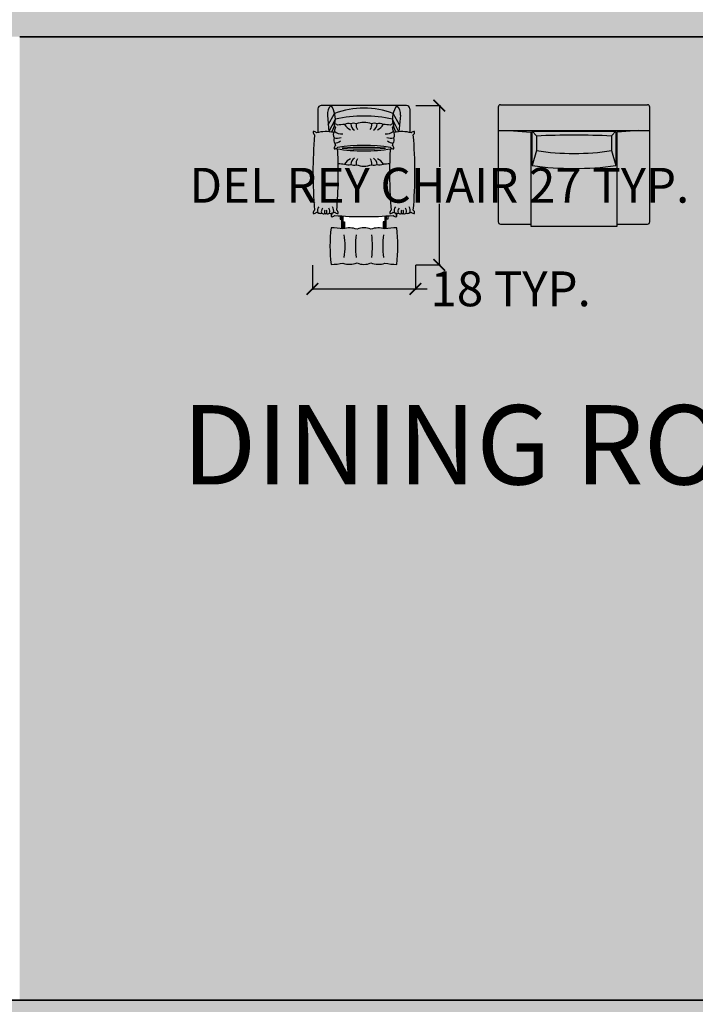
# Model space of a CAD drawing. Units: inches. Extents: x 1704 to 6393, y -157 to 1172.
# Tile 40 of 122: x 2081 to 2198, y 372 to 541. Entities that reach past the tile are written whole.
import ezdxf

# ---------------------------------------------------------------- set-up
doc = ezdxf.new("R2010")
doc.units = ezdxf.units.IN
doc.header["$MEASUREMENT"] = 0
for name, color, linetype, lineweight in [('A-ANNO-DIMS', 7, 'Continuous', 13), ('A-AREA-IDEN', 7, 'Continuous', 18), ('A-FURN', 8, 'Continuous', 18), ('A-WALL-PATT', 7, 'Continuous', 13), ('estofado', 7, 'Continuous', 25), ('WALLS', 7, 'Continuous', 35)]:
    doc.layers.add(name, color=color, linetype=linetype, lineweight=lineweight)
doc.layers.add('A-FLOR-PATT', color=7, linetype='Continuous', lineweight=13, true_color=0xf2f2f2)
doc.styles.get("Standard").update_dxf_attribs({"font": 'arial.ttf'})
doc.dimstyles.get("Standard").update_dxf_attribs({"dimtxt": 6, "dimasz": 2, "dimexe": 0.18, "dimexo": 0.0625, "dimgap": 0.09, "dimtad": 0, "dimtih": 1, "dimtoh": 1, "dimdec": 1, "dimzin": 0, "dimdsep": 46, "dimlunit": 3, "dimtxsty": 'Standard', "dimblk": 'ARCHTICK', "dimcen": 0.09, "dimadec": 0, "dimazin": 0, "dimtfac": 1, "dimtdec": 1, "dimtofl": 0, "dimtmove": 0, "dimatfit": 3, "dimfxl": 1, "dimtolj": 1, "dimtzin": 0, "dimarcsym": 0})

# ---------------------------------------------------------------- blocks, each defined once
blk = doc.blocks.new('Poltrona Del Rey Aliança')
at = {"layer": 'estofado', "ltscale": 0.1}
h = blk.add_hatch(color=256, dxfattribs=at)
h.dxf.hatch_style = 1
h.set_gradient(color1=(204, 209, 209), color2=(140, 151, 151), one_color=1, tint=0.57, name='CYLINDER')
h.paths.add_polyline_path([(-0.3291, -0.0872, -0.258328), (-0.295, 0), (-0.3837, 0, 0.414214), (-0.4137, -0.03), (-0.4137, -0.2425, -0.088666), (-0.3154, -0.2356)])
h.paths.add_polyline_path([(0.4137, -0.03, 0.414214), (0.3837, 0), (0.295, 0, -0.258328), (0.3291, -0.0872), (0.3154, -0.2356, -0.088666), (0.4137, -0.2425)])
h = blk.add_hatch(color=256, dxfattribs=at)
h.dxf.hatch_style = 1
h.set_gradient(color1=(204, 209, 209), color2=(140, 151, 151), one_color=1, tint=0.57, name='INVCYLINDER')
h.paths.add_polyline_path([(0.295, 0), (-0.295, 0, -0.089046), (-0.2635, -0.0705, -0.183028), (0.2635, -0.0705, -0.089046)])
h = blk.add_hatch(color=256, dxfattribs=at)
h.dxf.hatch_style = 1
h.set_gradient(color1=(204, 209, 209), color2=(140, 151, 151), one_color=1, tint=0.57)
h.paths.add_polyline_path([(-0.2635, -0.0705, 0.089046), (-0.295, 0, 0.258328), (-0.3291, -0.0872), (-0.3212, -0.1727)])
h.paths.add_polyline_path([(-0.2571, -0.1231, 0.060804), (-0.2635, -0.0705), (-0.3212, -0.1727), (-0.3154, -0.2356)])
h.paths.add_polyline_path([(-0.2655, -0.1833, -0.142988), (-0.2685, -0.1646, -0.055221), (-0.261, -0.1645, 0.047677), (-0.2571, -0.1231), (-0.3154, -0.2356, -0.022481), (-0.2906, -0.2393, 0.070542)])
h = blk.add_hatch(color=256, dxfattribs=at)
h.dxf.hatch_style = 1
h.set_gradient(color1=(204, 209, 209), color2=(140, 151, 151), one_color=1, tint=0.57, name='INVCYLINDER')
h.paths.add_polyline_path([(-0.2635, -0.0705, -0.060804), (-0.2571, -0.1231, -0.113324), (0.2571, -0.1231, -0.060804), (0.2635, -0.0705, 0.183028)])
h = blk.add_hatch(color=256, dxfattribs=at)
h.dxf.hatch_style = 1
h.set_gradient(color1=(204, 209, 209), color2=(140, 151, 151), one_color=1, tint=0.57)
h.paths.add_polyline_path([(0.295, 0, 0.089046), (0.2635, -0.0705), (0.3211, -0.1738), (0.3291, -0.0872, 0.258328)])
h.paths.add_polyline_path([(0.2635, -0.0705, 0.060804), (0.2571, -0.1231), (0.3154, -0.2356), (0.3211, -0.1738)])
h.paths.add_polyline_path([(0.2571, -0.1231, 0.047677), (0.261, -0.1645, -0.055221), (0.2685, -0.1646, -0.142988), (0.2655, -0.1833, 0.070542), (0.2906, -0.2393, -0.022481), (0.3154, -0.2356)])
h = blk.add_hatch(color=256, dxfattribs=at)
h.dxf.hatch_style = 1
h.set_gradient(color1=(204, 209, 209), color2=(85, 94, 94), one_color=1, tint=0.35, name='CURVED')
h.paths.add_polyline_path([(-0.2568, -0.1947, -0.107782), (-0.2655, -0.1833, -0.070542), (-0.2906, -0.2393, -0.016789), (-0.2722, -0.2436, -0.067663), (-0.2652, -0.2308, -0.033072)])
h.paths.add_polyline_path([(0.2571, -0.1231, 0.113324), (-0.2571, -0.1231, -0.047677), (-0.261, -0.1645, -0.196708), (-0.2383, -0.1763, -0.00792), (-0.1747, -0.1697, -0.182617), (-0.118, -0.1656, -0.204275), (-0.0697, -0.1634, -0.180654), (0.0697, -0.1634, -0.204275), (0.118, -0.1656, -0.182617), (0.1747, -0.1697, -0.00792), (0.2383, -0.1763, -0.196708), (0.261, -0.1645, -0.047677)])
h.paths.add_polyline_path([(0.2655, -0.1833, -0.107782), (0.2568, -0.1947, -0.033072), (0.2652, -0.2308, -0.067663), (0.2722, -0.2436, -0.016789), (0.2906, -0.2393, -0.070542)])
h = blk.add_hatch(color=256, dxfattribs=at)
h.dxf.hatch_style = 1
h.set_gradient(color1=(204, 209, 209), color2=(140, 151, 151), one_color=1, tint=0.57, name='INVCURVED')
h.paths.add_polyline_path([(0.2652, -0.2308, 0.033072), (0.2568, -0.1947, 0.254696), (0.2685, -0.1646, 0.254696), (0.2383, -0.1763, 0.00792), (0.1747, -0.1697, 0.182617), (0.118, -0.1656, 0.187401), (0.0735, -0.1621, 0.016251), (0.0697, -0.1634, 0.180654), (-0.0697, -0.1634, 0.204275), (-0.118, -0.1656, 0.263328), (-0.0893, -0.2185, -0.263328), (-0.118, -0.1656, 0.182617), (-0.1747, -0.1697, 0.00792), (-0.2383, -0.1763, 0.254696), (-0.2685, -0.1646, 0.254696), (-0.2568, -0.1947, 0.033072), (-0.2652, -0.2308, 0.299987), (-0.2685, -0.2905, 0.296972), (-0.2615, -0.3402, 0.016266), (-0.2568, -0.3578, 0.254696), (-0.2685, -0.388, 0.254696), (-0.2383, -0.3763, -0.073513), (0.2383, -0.3763, 0.254696), (0.2685, -0.388, 0.254696), (0.2568, -0.3578, 0.016266), (0.2615, -0.3402, 0.296972), (0.2685, -0.2905, 0.299987)])
h = blk.add_hatch(color=256, dxfattribs=at)
h.dxf.hatch_style = 1
h.set_gradient(color1=(204, 209, 209), one_color=1, tint=1)
h.paths.add_polyline_path([(-0.2358, -0.4039, 0.314303), (-0.2519, -0.386, -0.125347), (-0.2685, -0.388, -0.254696), (-0.2568, -0.3578, -0.016266), (-0.2615, -0.3402, -0.296972), (-0.2685, -0.2905, -0.227702), (-0.2722, -0.2436, 0.140506), (-0.4265, -0.2461, 0.254696), (-0.4567, -0.2344, 0.254696), (-0.445, -0.2646, 0.041763), (-0.445, -0.9409, 0.254696), (-0.4567, -0.971, 0.254696), (-0.4265, -0.9594, 0.011584), (-0.414, -0.9628, 0.212443), (-0.3803, -0.9693, 0.2364), (-0.3527, -0.9714, 0.216836), (-0.3417, -0.9734, 0.091294), (-0.3373, -0.9714, 0.2364), (-0.3097, -0.9693, 0.284493), (-0.3149, -0.9268, -0.284493), (-0.3097, -0.9693, 0.212443), (-0.276, -0.9628, 0.011584), (-0.2635, -0.9594, 0.254696), (-0.2333, -0.971, 0.254696), (-0.245, -0.9409, 0.033141)])
h = blk.add_hatch(color=256, dxfattribs=at)
h.dxf.hatch_style = 1
h.set_gradient(color1=(204, 209, 209), one_color=1, tint=1)
h.paths.add_polyline_path([(0.445, -0.2646, 0.254696), (0.4567, -0.2344, 0.254696), (0.4265, -0.2461, 0.140506), (0.2722, -0.2436, -0.227702), (0.2685, -0.2905, -0.296972), (0.2615, -0.3402, -0.016266), (0.2568, -0.3578, -0.254696), (0.2685, -0.388, -0.125347), (0.2519, -0.386, 0.314303), (0.2358, -0.4039, 0.033141), (0.245, -0.9409, 0.254696), (0.2333, -0.971, 0.254696), (0.2635, -0.9594, 0.011584), (0.276, -0.9628, 0.212443), (0.3097, -0.9693, 0.2364), (0.3373, -0.9714, 0.314353), (0.3527, -0.9714, 0.2364), (0.3803, -0.9693, 0.212443), (0.414, -0.9628, 0.011584), (0.4265, -0.9594, 0.254696), (0.4567, -0.971, 0.254696), (0.445, -0.9409, 0.041763)])
h = blk.add_hatch(color=256, dxfattribs=at)
h.dxf.hatch_style = 1
h.set_gradient(color1=(204, 209, 209), color2=(140, 151, 151), one_color=1, tint=0.57, name='INVCURVED')
h.paths.add_polyline_path([(-0.2383, -0.3763, -0.125347), (-0.2519, -0.386, -0.093275), (-0.2447, -0.3891, 0.075524), (0.2447, -0.3891, -0.093275), (0.2519, -0.386, -0.125347), (0.2383, -0.3763, 0.073513)])
h.paths.add_polyline_path([(0.1958, -0.3832, -0.03688), (-0.1958, -0.3832, -0.03688)], flags=16)
h = blk.add_hatch(color=256, dxfattribs=at)
h.dxf.hatch_style = 1
h.set_gradient(color1=(204, 209, 209), color2=(129, 141, 141), one_color=1, tint=0.53, name='CURVED')
h.paths.add_polyline_path([(0.2356, -0.4071, -0.253895), (0.2447, -0.3891, -0.075524), (-0.2447, -0.3891, -0.253895), (-0.2356, -0.4071, -0.006973), (-0.2317, -0.5201, 0.007144), (-0.1744, -0.5259, -0.00012), (-0.1743, -0.5259, 0.182617), (-0.1176, -0.53, 0.204275), (-0.0693, -0.5322, 0.180654), (0.0701, -0.5322, 0.204275), (0.1184, -0.53, 0.182617), (0.1751, -0.5259, 0.000052), (0.1751, -0.5258, 0.00705), (0.2317, -0.5201, -0.006973)])
h = blk.add_hatch(color=256, dxfattribs=at)
h.dxf.hatch_style = 1
h.set_gradient(color1=(204, 209, 209), one_color=1, tint=1, name='CYLINDER')
h.paths.add_polyline_path([(0.2317, -0.5201, -0.007042), (0.1752, -0.5258, -0.182811), (0.1184, -0.53, -0.204275), (0.0701, -0.5322, -0.180542), (-0.0693, -0.5323, -0.000018), (-0.0694, -0.5323, -0.203561), (-0.1175, -0.53, -0.000024), (-0.1177, -0.53, -0.181815), (-0.1742, -0.5259, -0.007163), (-0.2317, -0.5201, -0.025969), (-0.245, -0.9409, -0.254696), (-0.2333, -0.971, -0.254696), (-0.2635, -0.9594, -0.011584), (-0.276, -0.9628, -0.070407), (-0.2865, -0.9682, 0.130579), (-0.295, -0.9977), (-0.295, -1, 0.254696), (-0.2648, -0.9883, 0.044151), (0.2648, -0.9883, 0.254696), (0.295, -1), (0.295, -0.9977, 0.130579), (0.2865, -0.9682, -0.070407), (0.276, -0.9628, -0.011584), (0.2635, -0.9594, -0.254696), (0.2333, -0.971, -0.254696), (0.245, -0.9409, -0.025969)])
h = blk.add_hatch(color=256, dxfattribs=at)
h.dxf.hatch_style = 1
h.set_gradient(color1=(204, 209, 209), one_color=1, tint=1, name='CYLINDER')
h.paths.add_polyline_path([(0.295, -1.0999, 0.031185), (0.1884, -1.1106, 0.17196), (0.0623, -1.1138, 0.223433), (-0.0623, -1.1138, 0.17196), (-0.1884, -1.1106, 0.031185), (-0.295, -1.0999, 0.066975), (-0.295, -1.43, 0.031185), (-0.1884, -1.4193, 0.17196), (-0.0623, -1.4161, 0.223433), (0.0623, -1.4161, 0.17196), (0.1884, -1.4193, 0.031185), (0.295, -1.43, 0.066975)])
at = {"layer": 'estofado'}
for p, q in [((0.3837, 0), (-0.3837, 0)), ((-0.4137, -0.03), (-0.4137, -0.2425)), ((-0.3291, -0.0872), (-0.3154, -0.2356)), ((0.3291, -0.0872), (0.3154, -0.2356)), ((0.4137, -0.03), (0.4137, -0.2425)), ((-0.295, -0.9701), (-0.295, -1)), ((0.295, -1), (0.295, -0.9701))]:
    blk.add_line(p, q, dxfattribs=at)
at = {"layer": 'estofado', "ltscale": 0.1}
for p, q in [((-0.3212, -0.1727), (-0.2635, -0.0705)), ((0.3211, -0.1738), (0.2635, -0.0705)), ((-0.3154, -0.2356), (-0.2571, -0.1231)), ((0.3154, -0.2356), (0.2571, -0.1231))]:
    blk.add_line(p, q, dxfattribs=at)
for points in [[(-0.2141, -0.9924), (-0.2141, -1.0234), (-0.2033, -1.0234), (-0.2033, -0.9931)], [(-0.2003, -1.1087), (-0.2003, -0.9933)], [(-0.1897, -0.994), (-0.1897, -1.1104)], [(-0.1852, -1.1096), (-0.1852, -1.0474), (-0.1745, -1.0474), (-0.1745, -1.1066)], [(0.1852, -1.1096), (0.1852, -1.0474), (0.1745, -1.0474), (0.1745, -1.1066)], [(0.1897, -0.994), (0.1897, -1.1104)], [(0.2003, -1.1087), (0.2003, -0.9933)], [(0.2141, -0.9924), (0.2141, -1.0234), (0.2033, -1.0234), (0.2033, -0.9931)]]:
    blk.add_lwpolyline(points, dxfattribs=at)
at = {"layer": 'estofado'}
for centre, radius, start, end in [((-0.3837, -0.03), 0.03, 90, 180), ((-0.2333, -0.0744), 0.0967, 129.65366, 187.59148), ((-0.4756, -0.1231), 0.2185, 349.08151, 34.27248), ((0.4756, -0.1231), 0.2185, 145.72752, 190.91849), ((0.2333, -0.0744), 0.0967, 352.40852, 50.34634), ((0.3837, -0.03), 0.03, 360, 90), ((-0.2349, -0.1689), 0.0338, 172.61866, 229.77535), ((-0.2641, -0.1981), 0.0338, 40.22465, 97.38134), ((0, -2.1798), 2.0176, 94.96806, 96.78307), ((0, -2.1798), 2.0176, 83.21693, 85.03194), ((0.2641, -0.1981), 0.0338, 82.61866, 139.77535), ((0.2349, -0.1689), 0.0338, 310.22465, 7.38134), ((3.5965, -0.6027), 4.0556, 175.21711, 184.78289), ((-0.4232, -0.2388), 0.0338, 172.61866, 229.77535), ((-0.4524, -0.268), 0.0338, 40.22465, 97.38134), ((-0.345, -0.514), 0.28, 74.93962, 106.93174), ((-0.4756, -0.1231), 0.2185, 327.85602, 343.99631), ((-0.2215, -0.2632), 0.0544, 143.38498, 210.17914), ((0.0111, -0.2763), 0.28, 163.06826, 170.64501), ((-0.0111, -0.2763), 0.28, 9.35499, 16.93174), ((0.2215, -0.2632), 0.0544, 329.82086, 36.61502), ((0.4756, -0.1231), 0.2185, 196.00369, 212.14398), ((0.345, -0.514), 0.28, 73.06826, 105.06038), ((0.4524, -0.268), 0.0338, 82.61866, 139.77535), ((0.4232, -0.2388), 0.0338, 310.22465, 7.38134), ((-3.5965, -0.6027), 4.0556, 355.21711, 4.78289), ((-0.2269, -0.31), 0.046, 154.98172, 221.1415), ((0.0111, -0.2763), 0.28, 193.20412, 196.93174), ((-0.0111, -0.2763), 0.28, 343.06826, 346.79588), ((0.2269, -0.31), 0.046, 318.8585, 25.01828), ((-0.2349, -0.3836), 0.0338, 130.22465, 187.38134), ((-0.2641, -0.3545), 0.0338, 262.61866, 319.77535), ((-0.2567, -0.4065), 0.0211, 358.53397, 76.83372), ((-4.2865, -0.6027), 4.0556, 355.21711, 2.80978), ((0, -3.0337), 2.6577, 85.77582, 94.22418), ((0, 2.2673), 2.6577, 265.77582, 274.22418), ((4.2865, -0.6027), 4.0556, 177.19022, 184.78289), ((0.2567, -0.4065), 0.0211, 103.16628, 181.46603), ((0.2641, -0.3545), 0.0338, 220.22465, 277.38134), ((0.2349, -0.3836), 0.0338, 352.61866, 49.77535), ((0, 1.4842), 2.0176, 263.40516, 265.04688), ((0, 1.4842), 2.0176, 266.65527, 266.66071), ((0, 1.4842), 2.0176, 274.97902, 276.59484), ((0, 1.4842), 2.0176, 268.02834, 268.03255), ((-0.4232, -0.9667), 0.0338, 130.22465, 187.38134), ((-0.4524, -0.9375), 0.0338, 262.61866, 319.77535), ((-0.345, -0.6915), 0.28, 253.06826, 255.723), ((-0.2353, -0.9988), 0.0598, 149.12344, 181.11851), ((-0.345, -0.6915), 0.28, 284.277, 286.93174), ((-0.2376, -0.9375), 0.0338, 220.22465, 277.38134), ((-0.2668, -0.9667), 0.0338, 352.61866, 49.77535), ((0.2668, -0.9667), 0.0338, 130.22465, 187.38134), ((0.2376, -0.9375), 0.0338, 262.61866, 319.77535), ((0.345, -0.6915), 0.28, 253.06826, 255.723), ((0.2353, -0.9988), 0.0598, 358.88149, 30.87656), ((0.345, -0.6915), 0.28, 284.277, 286.93174), ((0.4524, -0.9375), 0.0338, 220.22465, 277.38134), ((0.4232, -0.9667), 0.0338, 352.61866, 49.77535), ((-0.2907, -0.9665), 0.0338, 262.61866, 319.77535), ((0, 2.0052), 3.0052, 264.94391, 275.05609), ((0.2907, -0.9665), 0.0338, 220.22465, 277.38134)]:
    blk.add_arc(centre, radius, start, end, dxfattribs=at)
at = {"layer": 'estofado', "ltscale": 0.1}
for centre, radius, start, end in [((0, -0.7661), 0.7439, 69.25617, 110.74383), ((0, -1.2427), 1.1487, 77.06919, 102.93081), ((-0.1409, -0.2427), 0.0805, 73.46231, 114.85878), ((-0.0792, -0.1148), 0.1102, 209.89617, 247.80825), ((-0.0912, -0.2211), 0.0616, 69.57655, 115.75748), ((-0.057, -0.1667), 0.061, 178.98456, 242.48365), ((-0.0035, -0.1761), 0.0675, 169.12551, 216.59576), ((0, -0.3501), 0.1993, 69.51952, 110.48048), ((0.0035, -0.1761), 0.0675, 323.40424, 10.87449), ((0.0912, -0.2211), 0.0616, 64.24252, 110.42345), ((0.057, -0.1667), 0.061, 297.51635, 1.01544), ((0.1409, -0.2427), 0.0805, 65.14122, 106.53769), ((0.0792, -0.1148), 0.1102, 292.19175, 330.10383), ((-0.2036, -0.1635), 0.0913, 227.53176, 278.05529), ((0.2036, -0.1635), 0.0913, 261.94471, 312.46824), ((-0.2431, -0.1831), 0.1104, 256.68043, 289.83371), ((-0.3064, -0.1722), 0.1739, 284.94614, 302.97426), ((0.2431, -0.1831), 0.1104, 250.16629, 283.31957), ((0.3064, -0.1722), 0.1739, 237.02574, 255.05386), ((0, 1.222), 1.6296, 261.36198, 278.63802), ((0, -1.9883), 1.6296, 81.59117, 98.40883), ((-0.0788, -0.5808), 0.1102, 112.19175, 150.10383), ((-0.1405, -0.4529), 0.0805, 245.14122, 286.53769), ((-0.0566, -0.5289), 0.061, 117.51635, 181.01544), ((-0.0908, -0.4745), 0.0616, 244.24252, 290.42345), ((-0.0031, -0.5195), 0.0675, 143.40424, 190.87449), ((0.0039, -0.5195), 0.0675, 349.12551, 36.59576), ((0.0916, -0.4745), 0.0616, 249.57655, 295.75748), ((0.0574, -0.5289), 0.061, 358.98456, 62.48365), ((0.1413, -0.4529), 0.0805, 253.46231, 294.85878), ((0.0796, -0.5808), 0.1102, 29.89617, 67.80825), ((0.0004, -0.3455), 0.1993, 249.51952, 290.48048), ((-0.369, -0.9438), 0.0489, 140.1555, 202.877), ((-0.3899, -0.9281), 0.0423, 235.25652, 283.23173), ((-0.3434, -0.9522), 0.0406, 137.80589, 204.86284), ((-0.3644, -0.9429), 0.0308, 238.98878, 292.19094), ((-0.3124, -0.9555), 0.0434, 159.33684, 201.47674), ((-0.345, -0.9603), 0.0135, 235.09864, 304.90136), ((-0.3776, -0.9555), 0.0434, 338.52326, 20.66316), ((-0.3256, -0.9429), 0.0308, 247.80906, 301.01122), ((-0.3466, -0.9522), 0.0406, 335.13716, 42.19411), ((-0.3001, -0.9281), 0.0423, 256.76827, 304.74348), ((-0.321, -0.9438), 0.0489, 337.123, 39.8445), ((0.321, -0.9438), 0.0489, 140.1555, 202.877), ((0.3001, -0.9281), 0.0423, 235.25652, 283.23173), ((0.3466, -0.9522), 0.0406, 137.80589, 204.86284), ((0.3256, -0.9429), 0.0308, 238.98878, 292.19094), ((0.3776, -0.9555), 0.0434, 159.33684, 201.47674), ((0.345, -0.9603), 0.0135, 235.09864, 304.90136), ((0.3124, -0.9555), 0.0434, 338.52326, 20.66316), ((0.3644, -0.9429), 0.0308, 247.80906, 301.01122), ((0.3434, -0.9522), 0.0406, 335.13716, 42.19411), ((0.3899, -0.9281), 0.0423, 256.76827, 304.74348), ((0.369, -0.9438), 0.0489, 337.123, 39.8445), ((0.9317, -1.2649), 1.2378, 172.33668, 187.66332), ((-0.3276, -1.9587), 0.8594, 80.68246, 87.82718), ((-0.1299, -1.2902), 0.1889, 69.03471, 108.06338), ((0, -1.2462), 0.1463, 64.81025, 115.18975), ((0.1299, -1.2902), 0.1889, 71.93662, 110.96529), ((0.3276, -1.9587), 0.8594, 92.17282, 99.31754), ((-0.9317, -1.2649), 1.2378, 352.33668, 7.66332), ((-0.8046, -1.2649), 0.6352, 350.72425, 9.27575), ((0.7218, -1.2649), 0.7985, 172.63295, 187.36705), ((-0.7218, -1.2649), 0.7985, 352.63295, 7.36705), ((0.8046, -1.2649), 0.6352, 170.72425, 189.27575), ((-0.1299, -1.2397), 0.1889, 251.93662, 290.96529), ((0, -1.2837), 0.1463, 244.81025, 295.18975), ((0.1299, -1.2397), 0.1889, 249.03471, 288.06338), ((-0.3276, -0.5712), 0.8594, 272.17282, 279.31754), ((0.3276, -0.5712), 0.8594, 260.68246, 267.82718)]:
    blk.add_arc(centre, radius, start, end, dxfattribs=at)
blk = doc.blocks.new('poltrona biquisten 2')
at = {"layer": 'estofado', "ltscale": 0.5}
h = blk.add_hatch(color=256, dxfattribs=at)
h.dxf.hatch_style = 1
h.set_gradient(color1=(165, 192, 175), color2=(222, 232, 226), one_color=1, tint=0.89, name='INVCURVED')
h.paths.add_polyline_path([(0.65, 1.02, 0.414214), (0.63, 1.04), (-0.63, 1.04, 0.414214), (-0.65, 1.02), (-0.65, 0.82), (0.65, 0.82)])
h = blk.add_hatch(color=256, dxfattribs=at)
h.dxf.hatch_style = 1
h.set_gradient(color1=(165, 192, 175), color2=(222, 232, 226), one_color=1, tint=0.89)
h.paths.add_polyline_path([(-0.37, 0.8064), (-0.5562, 0.82), (-0.65, 0.82), (-0.65, 0.0379, 0.414214), (-0.63, 0.0179), (-0.37, 0.0179)])
h = blk.add_hatch(color=256, dxfattribs=at)
h.dxf.hatch_style = 1
h.set_gradient(color1=(165, 192, 175), color2=(222, 232, 226), one_color=1, tint=0.89, name='INVCURVED')
h.paths.add_polyline_path([(0.37, 0.8064), (0.5562, 0.82), (-0.5562, 0.82), (-0.37, 0.8064), (-0.37, 0), (0.37, 0)])
h.paths.add_polyline_path([(-0.3585, 0.5186), (-0.3585, 0.8144), (0.3585, 0.8144), (0.3585, 0.5186, -0.068679)], flags=16)
h.paths.add_polyline_path([(-0.3207, 0.6475), (-0.3207, 0.7727, -0.023546), (0.3207, 0.7727), (0.3207, 0.6475, -0.077277)], flags=0)
h = blk.add_hatch(color=256, dxfattribs=at)
h.dxf.hatch_style = 1
h.set_gradient(color1=(165, 192, 175), color2=(222, 232, 226), one_color=1, tint=0.89, name='CYLINDER')
h.paths.add_polyline_path([(0.3585, 0.8144), (-0.3585, 0.8144), (-0.3207, 0.7727, -0.023546), (0.3207, 0.7727)])
h = blk.add_hatch(color=256, dxfattribs=at)
h.dxf.hatch_style = 1
h.set_gradient(color1=(165, 192, 175), color2=(222, 232, 226), one_color=1, tint=0.89, name='CYLINDER')
h.paths.add_polyline_path([(-0.3207, 0.7727), (-0.3585, 0.8144), (-0.3585, 0.5186), (-0.3207, 0.6475)])
h.paths.add_polyline_path([(0.3585, 0.8144), (0.3207, 0.7727), (0.3207, 0.6475), (0.3585, 0.5186)])
h.paths.add_polyline_path([(0.3207, 0.6475, -0.077277), (-0.3207, 0.6475), (-0.3585, 0.5186, 0.068679), (0.3585, 0.5186)])
h = blk.add_hatch(color=256, dxfattribs=at)
h.dxf.hatch_style = 1
h.set_gradient(color1=(165, 192, 175), color2=(222, 232, 226), one_color=1, tint=0.89, name='INVCURVED')
h.paths.add_polyline_path([(0.3207, 0.7727, 0.023546), (-0.3207, 0.7727), (-0.3207, 0.6475, 0.077277), (0.3207, 0.6475)])
h = blk.add_hatch(color=256, dxfattribs=at)
h.dxf.hatch_style = 1
h.set_gradient(color1=(165, 192, 175), color2=(222, 232, 226), one_color=1, tint=0.89)
h.paths.add_polyline_path([(0.65, 0.82), (0.5562, 0.82), (0.37, 0.8064), (0.37, 0.0179), (0.63, 0.0179, 0.414214), (0.65, 0.0379)])
for p, q in [((-0.65, 1.02), (-0.65, 0.0379)), ((-0.63, 1.04), (0.63, 1.04)), ((0.65, 0.0379), (0.65, 1.02)), ((-0.65, 0.82), (0.65, 0.82)), ((-0.5562, 0.82), (-0.37, 0.8064)), ((-0.37, 0.8064), (-0.37, 0)), ((-0.3585, 0.8144), (-0.3207, 0.7727)), ((-0.3207, 0.7727), (-0.3207, 0.6475)), ((0.3585, 0.8144), (0.3207, 0.7727)), ((0.3207, 0.7727), (0.3207, 0.6475)), ((0.5562, 0.82), (0.37, 0.8064)), ((0.37, 0), (0.37, 0.8064)), ((-0.3207, 0.6475), (-0.3585, 0.5186)), ((0.3207, 0.6475), (0.3585, 0.5186)), ((-0.63, 0.0179), (-0.37, 0.0179)), ((-0.37, 0), (0.37, 0)), ((0.37, 0.0179), (0.63, 0.0179))]:
    blk.add_line(p, q, dxfattribs=at)
blk.add_lwpolyline([(-0.3585, 0.5186), (-0.3585, 0.8144), (0.3585, 0.8144), (0.3585, 0.5186)], dxfattribs=at)
for centre, radius, start, end in [((-0.63, 1.02), 0.02, 90, 180), ((0.63, 1.02), 0.02, 0, 90), ((0, -6.0334), 6.8136, 87.3023, 92.6977), ((0, 2.7101), 2.0874, 261.16232, 278.83768), ((0, 3.1159), 2.6219, 262.14225, 277.85775), ((-0.63, 0.0379), 0.02, 180, 270), ((0.63, 0.0379), 0.02, 270, 0)]:
    blk.add_arc(centre, radius, start, end, dxfattribs=at)
blk = doc.blocks.new('_ArchTick')
at = {"color": 0, "linetype": 'ByBlock', "const_width": 0.15}
blk.add_lwpolyline([(-0.5, -0.5), (0.5, 0.5)], dxfattribs=at)
blk = doc.blocks.new('*D60')
at = {"layer": 'A-ANNO-DIMS', "color": 0, "lineweight": -2, "transparency": 16777216}
for p, q in [((2149.61, 526.36), (2153.85, 526.36)), ((2153.67, 526.36), (2153.67, 515.83)), ((2153.67, 498.91), (2153.67, 509.44)), ((2149.61, 498.91), (2153.85, 498.91))]:
    blk.add_line(p, q, dxfattribs=at)
at = {"layer": 'Defpoints', "color": 0, "lineweight": -3, "transparency": 16777216}
for p in [(2149.55, 526.36), (2153.67, 526.36), (2149.55, 498.91)]:
    blk.add_point(p, dxfattribs=at)
at = {"layer": 'A-ANNO-DIMS', "color": 0, "lineweight": -2, "transparency": 16777216, "xscale": 2, "yscale": 2, "zscale": 2}
for p, rotation in [((2153.67, 526.36), 90), ((2153.67, 498.91), 270)]:
    blk.add_blockref('_ArchTick', p, dxfattribs=dict(at, rotation=rotation))
at = {"layer": 'A-ANNO-DIMS', "color": 0, "transparency": 16777216, "insert": (2153.67, 512.63), "char_height": 6, "attachment_point": 5}
blk.add_mtext('\\A1;DEL REY CHAIR 27 TYP.', dxfattribs=at)
blk = doc.blocks.new('*D61')
at = {"layer": 'A-ANNO-DIMS', "color": 0, "lineweight": -2, "transparency": 16777216}
for p, q in [((2131.8, 498.85), (2131.8, 494.61)), ((2149.55, 498.85), (2149.55, 494.61)), ((2131.8, 494.79), (2149.55, 494.79)), ((2149.55, 494.79), (2151.55, 494.79))]:
    blk.add_line(p, q, dxfattribs=at)
at = {"layer": 'Defpoints', "color": 0, "lineweight": -3, "transparency": 16777216}
for p in [(2131.8, 498.91), (2149.55, 498.91), (2149.55, 494.79)]:
    blk.add_point(p, dxfattribs=at)
at = {"layer": 'A-ANNO-DIMS', "color": 0, "lineweight": -2, "transparency": 16777216, "xscale": 2, "yscale": 2, "zscale": 2, "rotation": 180}
blk.add_blockref('_ArchTick', (2131.8, 494.79), dxfattribs=at)
at = {"layer": 'A-ANNO-DIMS', "color": 0, "lineweight": -2, "transparency": 16777216, "xscale": 2, "yscale": 2, "zscale": 2}
blk.add_blockref('_ArchTick', (2149.55, 494.79), dxfattribs=at)
at = {"layer": 'A-ANNO-DIMS', "color": 0, "transparency": 16777216, "insert": (2165.96, 494.79), "char_height": 6, "attachment_point": 5}
blk.add_mtext('\\A1;18 TYP.', dxfattribs=at)
blk = doc.blocks.new('*D93')
at = {"layer": 'A-ANNO-DIMS', "color": 0, "lineweight": -2, "transparency": 16777216}
for p, q in [((2605.29, 895.21), (1829.7, 895.21)), ((1829.88, 895.21), (1829.88, 495.87)), ((1829.88, 90.21), (1829.88, 489.56)), ((2605.29, 90.21), (1829.7, 90.21))]:
    blk.add_line(p, q, dxfattribs=at)
at = {"layer": 'Defpoints', "color": 0, "lineweight": -3, "transparency": 16777216}
for p in [(2605.35, 895.21), (1829.88, 90.21), (2605.35, 90.21)]:
    blk.add_point(p, dxfattribs=at)
at = {"layer": 'A-ANNO-DIMS', "color": 0, "lineweight": -2, "transparency": 16777216, "xscale": 2, "yscale": 2, "zscale": 2}
for p, rotation in [((1829.88, 895.21), 90), ((1829.88, 90.21), 270)]:
    blk.add_blockref('_ArchTick', p, dxfattribs=dict(at, rotation=rotation))
at = {"layer": 'A-ANNO-DIMS', "color": 0, "transparency": 16777216, "insert": (1829.88, 492.71), "char_height": 6, "attachment_point": 5}
blk.add_mtext('\\A1;805', dxfattribs=at)

msp = doc.modelspace()

# ---------------------------------------------------------------- hatches: boundary and pattern name
at = {"layer": 'A-FLOR-PATT', "transparency": 33554528}
h = msp.add_hatch(color=256, dxfattribs=at)
h.dxf.hatch_style = 1
h.paths.add_polyline_path([(2273.349, 538.213), (2081.349, 538.213), (2081.349, 372.213), (2273.349, 372.213)])
h.paths.add_polyline_path([(2189.542, 505.951), (2184.316, 505.951), (2184.316, 505.591), (2169.442, 505.591), (2169.442, 505.951), (2164.216, 505.951, -0.4142136), (2163.814, 506.353), (2163.814, 526.093, -0.4142136), (2164.216, 526.495), (2189.542, 526.495, -0.4142136), (2189.944, 526.093), (2189.944, 506.353, -0.4142136)], flags=16)
h.paths.add_polyline_path([(2200.535, 511.491), (2200.535, 526.191), (2217.621, 526.191), (2217.621, 511.491), (2214.605, 511.491, -0.3946213), (2214.203, 511.116), (2203.952, 511.116, -0.3946213), (2203.551, 511.491)], flags=16)
h.paths.add_polyline_path([(2200.736, 511.692), (2200.736, 525.99), (2203.55, 525.99), (2203.55, 523.838, 0.1045605), (2214.605, 523.838), (2214.605, 525.99), (2217.42, 525.99), (2217.42, 511.692), (2214.605, 511.692), (2214.605, 523.838, -0.1045605), (2203.55, 523.838), (2203.55, 511.692)], flags=0)
h.paths.add_polyline_path([(2203.952, 511.317, -0.4142136), (2203.751, 511.518), (2203.751, 523.591, 0.099912), (2214.404, 523.591), (2214.404, 511.518, -0.4142136), (2214.203, 511.317)], flags=0)
h.paths.add_polyline_path([(2184.084, 516.015, -0.0686795), (2169.674, 516.015), (2169.674, 522.073), (2184.084, 522.073)], flags=0)
h.paths.add_polyline_path([(2183.325, 518.606, -0.0772766), (2170.433, 518.606), (2170.433, 521.123, -0.0235462), (2183.325, 521.123)], flags=0)
h.paths.add_polyline_path([(2135.029, 507.225, -0.1405189), (2135.191, 507.834, -0.0513838), (2135.029, 507.797)], flags=16)
h.paths.add_polyline_path([(2146.318, 498.997, -0.0311848), (2144.279, 499.202, -0.1719602), (2141.865, 499.263, -0.2234326), (2139.482, 499.263, -0.1719602), (2137.068, 499.202, -0.0311848), (2135.029, 498.997, -0.066975), (2135.029, 505.313, -0.0276914), (2136.841, 505.144), (2136.841, 506.777), (2136.576, 506.777), (2136.576, 507.371, 0.039911), (2145.741, 507.448, 0.2546956), (2146.318, 507.225), (2146.318, 507.269, 0.1305786), (2146.156, 507.834, -0.0704067), (2145.953, 507.935, -0.011584), (2145.714, 508.002, -0.2546956), (2145.137, 507.779, -0.2546956), (2145.361, 508.355, -0.0259693), (2145.107, 516.407, -0.0070422), (2144.025, 516.297, -0.1828112), (2142.939, 516.218, -0.2042746), (2142.015, 516.175, -0.1805419), (2139.348, 516.174, -0.0000184), (2139.345, 516.174, -0.2035615), (2138.425, 516.217, -0.0000237), (2138.421, 516.217, -0.1818152), (2137.34, 516.296, -0.0071635), (2136.24, 516.407, 0.007166), (2136.162, 518.63, 0.314303), (2135.854, 518.974, -0.1253469), (2135.537, 518.935, -0.2546956), (2135.76, 519.512, -0.0162662), (2135.67, 519.849, -0.296972), (2135.535, 520.8, -0.227702), (2135.464, 521.698, 0.1283977), (2132.757, 521.718), (2132.757, 525.785, -0.4142136), (2133.331, 526.359), (2148.015, 526.359, -0.4142136), (2148.589, 525.785), (2148.589, 521.718, -0.0118936), (2148.835, 521.65, -0.2546956), (2149.412, 521.873, -0.2546956), (2149.188, 521.296, -0.0417628), (2149.188, 508.355, -0.2546956), (2149.412, 507.779, -0.2546956), (2148.835, 508.002, -0.011584), (2148.596, 507.935, -0.2124435), (2147.949, 507.813, -0.2363999), (2147.423, 507.772, -0.3143526), (2147.126, 507.772, -0.2363999), (2146.6, 507.813, -0.0879275), (2146.318, 507.797), (2146.318, 507.225, -0.2546956), (2145.741, 507.448, -0.0042329), (2144.771, 507.371), (2144.771, 506.777), (2144.506, 506.777), (2144.506, 505.144, -0.0276914), (2146.318, 505.313, -0.066975)], flags=16)
h.paths.add_polyline_path([(2141.865, 505.047, 0.2234326), (2139.482, 505.047, 0.1738145), (2137.043, 505.1), (2137.043, 506.317), (2137.335, 506.317), (2137.335, 505.184, -0.1522072), (2139.482, 505.047, -0.2234326), (2141.865, 505.047, -0.1522072), (2144.011, 505.184), (2144.011, 506.317), (2144.304, 506.317), (2144.304, 505.1, 0.1738145)], flags=0)
h.paths.add_polyline_path([(2145.233, 522.986, 0.0079197), (2144.017, 523.111, 0.1826165), (2142.931, 523.19, 0.2042746), (2142.008, 523.233, 0.1806536), (2139.339, 523.233, 0.2042746), (2138.415, 523.19, 0.1826165), (2137.33, 523.111, 0.0079197), (2136.114, 522.986, 0.1967082), (2135.679, 523.212, 0.047677), (2135.755, 524.004), (2134.638, 521.852), (2134.376, 524.691, -0.2583282), (2135.029, 526.359, -0.0890464), (2135.632, 525.01, -0.1830277), (2145.715, 525.01, -0.0890464), (2146.318, 526.359, -0.2583282), (2146.971, 524.691), (2146.709, 521.852), (2145.592, 524.004, 0.047677), (2145.668, 523.212, 0.1967082)], flags=0)
h.paths.add_polyline_path([(2144.419, 519.027, -0.0368796), (2136.927, 519.027, -0.0368796)], flags=0)
h.paths.add_polyline_path([(2273.349, 629.213), (2213.349, 629.213), (2213.349, 573.213), (2213.349, 545.213), (2273.349, 545.213)])
h.paths.add_polyline_path([(2273.349, 711.213), (2207.349, 711.213), (2207.349, 709.213), (2231.349, 709.213), (2231.349, 707.213), (2207.349, 707.213), (2207.349, 631.213), (2273.349, 631.213)])
h.paths.add_polyline_path([(2273.349, 364.213), (2081.349, 364.213), (2081.349, 202.213), (2225.349, 202.213), (2229.181, 202.213), (2230.482, 202.213), (2268.215, 202.213), (2269.516, 202.213), (2273.349, 202.213)])
h.paths.add_polyline_path([(2203.551, 339.558, 0.3946213), (2203.952, 339.183), (2214.203, 339.183), (2214.203, 339.384), (2203.751, 339.384), (2203.751, 339.558)], flags=16)
h.paths.add_polyline_path([(2203.55, 351.7), (2203.55, 339.759), (2200.535, 339.759), (2200.535, 354.258), (2217.621, 354.258), (2217.621, 339.558), (2214.404, 339.558), (2214.404, 351.659, -0.101837)], flags=16)
h.paths.add_polyline_path([(2214.404, 354.057), (2214.605, 354.057), (2214.605, 354.258), (2214.404, 354.258)], flags=16)
h.paths.add_polyline_path([(2189.542, 334.018), (2184.316, 334.018), (2184.316, 333.658), (2169.442, 333.658), (2169.442, 334.018), (2164.216, 334.018, -0.4142136), (2163.814, 334.42), (2163.814, 354.161, -0.4142136), (2164.216, 354.563), (2189.542, 354.563, -0.4142136), (2189.944, 354.161), (2189.944, 334.42, -0.4142136)], flags=16)
h.paths.add_polyline_path([(2184.084, 344.083, -0.0686795), (2169.674, 344.083), (2169.674, 349.85), (2165.7, 350.14), (2188.058, 350.14), (2184.084, 349.85)], flags=0)
h.paths.add_polyline_path([(2183.325, 346.673, -0.0772766), (2170.433, 346.673), (2170.433, 349.19, -0.0235462), (2183.325, 349.19)], flags=0)
h.paths.add_polyline_path([(2134.638, 349.919), (2134.376, 352.758, -0.2583282), (2135.029, 354.426), (2133.331, 354.426, 0.4142136), (2132.757, 353.852), (2132.757, 349.785, -0.0886664)], flags=16)
h.paths.add_polyline_path([(2136.114, 351.053, -0.0079197), (2137.33, 351.178, -0.1826165), (2138.415, 351.257, -0.2042746), (2139.339, 351.3, -0.1806536), (2142.008, 351.3, -0.2042746), (2142.931, 351.257, -0.1826165), (2144.017, 351.178, -0.0079197), (2145.233, 351.053, -0.1967082), (2145.668, 351.279, -0.047677), (2145.592, 352.071, 0.1133241), (2135.755, 352.071, -0.047677), (2135.679, 351.279, -0.1967082)], flags=16)
h.paths.add_polyline_path([(2145.184, 346.697, 0.0331414), (2145.361, 336.423, 0.2546956), (2145.137, 335.846, 0.3030408), (2145.781, 336.164, 0.2903634), (2146.6, 335.88, 0.2363999), (2147.126, 335.839, -0.280712), (2147.275, 336.69, -0.280712), (2147.423, 335.839, 0.2363999), (2147.949, 335.88, 0.2903634), (2148.768, 336.164, 0.3030408), (2149.412, 335.846, 0.2546956), (2149.188, 336.423, 0.0417628), (2149.188, 349.363, 0.2546956), (2149.412, 349.94, 0.2546956), (2148.835, 349.717, 0.1405058), (2145.883, 349.765, -0.227702), (2145.812, 348.867, -0.296972), (2145.677, 347.916, -0.0162662), (2145.586, 347.579, -0.2546956), (2145.81, 347.002, -0.1253469), (2145.493, 347.041, 0.314303)], flags=16)
h.paths.add_polyline_path([(2135.029, 335.292, -0.1405189), (2135.191, 335.901, -0.1399435), (2134.747, 335.88, -0.2363999), (2134.22, 335.839, -0.3143526), (2133.924, 335.839, -0.280712), (2134.072, 336.69, -0.280712), (2134.22, 335.839, 0.2363999), (2134.747, 335.88, 0.2903634), (2135.566, 336.164, 0.3030408), (2136.209, 335.846, 0.2546956), (2135.985, 336.423, 0.0331414), (2136.162, 346.697, 0.314303), (2135.854, 347.041, -0.1253469), (2135.537, 347.002, -0.2546956), (2135.76, 347.579, -0.0162662), (2135.67, 347.916, -0.296972), (2135.535, 348.867, -0.2999866), (2135.599, 350.01, -0.0330719), (2135.76, 350.7, -0.3502076), (2135.604, 351.492), (2134.638, 349.919), (2135.604, 351.492, 0.3502076), (2135.76, 350.7, 0.0330719), (2135.599, 350.01, 0.2999866), (2135.535, 348.867, 0.296972), (2135.67, 347.916, 0.0279375), (2135.971, 347.698, 0.3576436), (2135.537, 347.002, 0.1253469), (2135.854, 347.041, -0.3555912), (2136.165, 346.637, -0.0329482), (2135.985, 336.423, -0.2546956), (2136.209, 335.846, -0.2546956), (2135.632, 336.069, -0.011584), (2135.393, 336.003, -0.1222327), (2135.029, 335.864)], flags=16)
h.paths.add_polyline_path([(2136.841, 335.42), (2136.783, 335.423), (2136.783, 334.844), (2136.841, 334.471)], flags=16)
h.paths.add_polyline_path([(2146.318, 327.064, -0.0311848), (2144.279, 327.269, -0.1719602), (2141.865, 327.33, -0.2234326), (2139.482, 327.33, -0.1719602), (2137.068, 327.269, -0.0311848), (2135.029, 327.064, -0.066975), (2135.029, 333.38, -0.0311848), (2137.068, 333.175, -0.1719602), (2139.482, 333.114, -0.2234326), (2141.865, 333.114, -0.1522072), (2144.011, 333.251), (2144.011, 334.384), (2144.304, 335.406, 0.0020345), (2144.771, 335.438), (2144.771, 334.844), (2144.506, 333.211, -0.0276914), (2146.318, 333.38, -0.066975)], flags=16)
h.paths.add_polyline_path([(2137.129, 334.384), (2137.335, 334.384), (2137.335, 333.251), (2137.129, 333.195)], flags=16)
h.paths.add_polyline_path([(2144.419, 347.094, -0.0368796), (2136.927, 347.094, -0.0368796)], flags=16)
at = {"layer": 'A-WALL-PATT', "transparency": 33554643}
h = msp.add_hatch(color=256, dxfattribs=at)
h.dxf.hatch_style = 1
h.paths.add_polyline_path([(2167.349, 895.213), (2073.349, 895.213), (2073.349, 887.213), (2081.349, 887.213), (2167.349, 887.213)])
h.paths.add_polyline_path([(2465.349, 895.213), (2273.349, 895.213), (2273.349, 903.213), (2263.349, 903.213), (2263.349, 895.213), (2263.349, 887.213), (2325.349, 887.213), (2325.349, 863.213), (2333.349, 863.213), (2333.349, 887.213), (2465.349, 887.213)])
h.paths.add_polyline_path([(2533.349, 895.213), (2513.349, 895.213), (2513.349, 887.213), (2513.349, 861.213), (2517.349, 861.213), (2517.349, 887.213), (2533.349, 887.213)])
h.paths.add_polyline_path([(2605.349, 895.213), (2581.349, 895.213), (2581.349, 887.213), (2597.349, 887.213), (2597.349, 854.213), (2605.349, 854.213)])
h.paths.add_polyline_path([(2605.349, 752.213), (2629.349, 752.213), (2629.349, 716.213), (2605.349, 716.213), (2605.349, 712.213), (2719.349, 712.213), (2719.349, 716.213), (2631.349, 716.213), (2631.349, 754.213), (2605.349, 754.213), (2605.349, 794.213), (2597.349, 794.213), (2597.349, 787.213), (2517.349, 787.213), (2517.349, 813.213), (2513.349, 813.213), (2513.349, 783.213), (2517.349, 783.213), (2597.349, 783.213), (2597.349, 719.213), (2517.349, 719.213), (2517.349, 753.213), (2513.349, 753.213), (2513.349, 719.213), (2365.349, 719.213), (2365.349, 763.213), (2325.349, 763.213), (2325.349, 755.213), (2357.349, 755.213), (2357.349, 719.213), (2325.349, 719.213), (2325.349, 711.213), (2547.349, 711.213), (2547.349, 615.213), (2449.349, 615.213), (2449.349, 607.213), (2514.349, 607.213), (2514.349, 546.213), (2439.349, 546.213), (2425.349, 546.213), (2425.349, 607.213), (2425.349, 615.213), (2350.349, 615.213), (2350.349, 589.713), (2358.349, 589.713), (2358.349, 610.213), (2420.349, 610.213), (2420.349, 545.213), (2358.349, 545.213), (2358.349, 565.713), (2350.349, 565.713), (2350.349, 538.213), (2469.349, 538.213), (2469.349, 459.213), (2469.349, 372.213), (2423.349, 372.213), (2423.349, 364.213), (2473.349, 364.213), (2473.349, 318.213), (2477.349, 318.213), (2477.349, 364.213), (2547.349, 364.213), (2547.349, 352.213), (2549.349, 352.213), (2549.349, 364.213), (2597.349, 364.213), (2597.349, 328.213), (2549.349, 328.213), (2547.349, 328.213), (2547.349, 326.213), (2549.349, 326.213), (2597.349, 326.213), (2605.349, 326.213), (2605.349, 377.057), (2597.349, 377.057), (2597.349, 372.213), (2477.349, 372.213), (2477.349, 451.213), (2597.349, 451.213), (2605.349, 451.213), (2605.349, 459.213), (2597.349, 459.213), (2477.349, 459.213), (2477.349, 538.213), (2597.349, 538.213), (2597.349, 495.213), (2605.349, 495.213), (2605.349, 512.213), (2631.349, 512.213), (2631.349, 568.213), (2605.349, 568.213), (2605.349, 577.213), (2597.349, 577.213), (2597.349, 542.213), (2518.349, 542.213), (2518.349, 607.213), (2532.349, 607.213), (2605.349, 607.213), (2605.349, 615.213), (2597.349, 615.213), (2551.349, 615.213), (2551.349, 711.213), (2597.349, 711.213), (2597.349, 645.213), (2605.349, 645.213), (2605.349, 712.213), (2605.349, 716.213)])
h.paths.add_polyline_path([(2605.349, 566.213), (2629.349, 566.213), (2629.349, 514.213), (2605.349, 514.213)], flags=16)
h.paths.add_polyline_path([(2381.349, 372.213), (2349.349, 372.213), (2349.349, 202.213), (2337.349, 202.213), (2337.349, 194.213), (2349.349, 194.213), (2349.349, 90.213), (2349.349, 72.213), (2357.349, 72.213), (2357.349, 90.213), (2381.349, 90.213), (2381.349, 98.213), (2357.349, 98.213), (2357.349, 266.213), (2381.349, 266.213), (2381.349, 270.213), (2353.349, 270.213), (2353.349, 364.213), (2381.349, 364.213)])
h.paths.add_polyline_path([(2605.349, 302.213), (2597.349, 302.213), (2597.349, 270.213), (2477.349, 270.213), (2477.349, 294.213), (2473.349, 294.213), (2473.349, 270.213), (2423.349, 270.213), (2423.349, 266.213), (2597.349, 266.213), (2597.349, 218.213), (2605.349, 218.213)])
h.paths.add_polyline_path([(2605.349, 146.213), (2597.349, 146.213), (2597.349, 98.213), (2429.349, 98.213), (2429.349, 90.213), (2597.349, 90.213), (2597.349, 72.213), (2605.349, 72.213), (2605.349, 90.213)])
h.paths.add_polyline_path([(2225.349, 202.213), (2049.349, 202.213), (2049.349, 194.213), (2225.349, 194.213)])
h.paths.add_polyline_path([(2289.349, 202.213), (2277.349, 202.213), (2273.349, 202.213), (2269.516, 202.213), (2269.516, 194.213), (2273.349, 194.213), (2277.349, 194.213), (2289.349, 194.213)])
h.paths.add_polyline_path([(2273.349, 372.213), (2029.19, 372.213), (2029.19, 364.213), (2273.349, 364.213)])
h.paths.add_polyline_path([(2277.349, 545.213), (2213.349, 545.213), (2213.349, 573.213), (2205.349, 573.213), (2177.349, 573.213), (2177.349, 545.213), (2073.349, 545.213), (2073.349, 538.213), (2081.349, 538.213), (2277.349, 538.213)])
h.paths.add_polyline_path([(2181.349, 545.213), (2181.349, 569.213), (2205.349, 569.213), (2205.349, 545.213)], flags=16)
h.paths.add_polyline_path([(2277.349, 719.213), (2081.349, 719.213), (2073.349, 719.213), (2073.349, 711.213), (2154.575, 711.213), (2205.349, 711.213), (2205.349, 687.213), (2205.349, 629.213), (2213.349, 629.213), (2273.349, 629.213), (2273.349, 631.213), (2207.349, 631.213), (2207.349, 707.213), (2231.349, 707.213), (2231.349, 709.213), (2207.349, 709.213), (2207.349, 711.213), (2277.349, 711.213)])

# ---------------------------------------------------------------- linework, layer by layer
at = {"layer": 'WALLS'}
for p, q in [((2277.349, 538.213), (2081.349, 538.213)), ((2277.349, 372.213), (2029.19, 372.213))]:
    msp.add_line(p, q, dxfattribs=at)

# ---------------------------------------------------------------- block references
at = {"layer": 'A-FURN'}
for name, p, xscale, yscale, zscale in [('Poltrona Del Rey Aliança', (2140.673, 526.359), 19.13431682689143, 19.13431682689143, 19.13431682689143), ('poltrona biquisten 2', (2176.879, 505.591), 20.10025524054769, 20.10025524054769, 20.10025524054769)]:
    msp.add_blockref(name, p, dxfattribs=dict(at, xscale=xscale, yscale=yscale, zscale=zscale))

# ---------------------------------------------------------------- texts
at = {"layer": 'A-AREA-IDEN'}
msp.add_text('DINING ROOM', height=13.6672, dxfattribs=at).set_placement((2109.317, 461.082))

# ---------------------------------------------------------------- dimensions: what is measured, and where the dimension line sits
at = {"layer": 'A-ANNO-DIMS'}
dim = msp.add_linear_dim(base=(1829.878, 90.213), p1=(2605.349, 895.213), p2=(2605.349, 90.213), angle=90, dimstyle='Standard', override={"dimdec": 0, "dimlfac": 1, "dimrnd": 0, "dimzin": 0, "dimdsep": 46, "dimlunit": 2}, dxfattribs=at)
dim.commit()
dim.dimension.update_dxf_attribs({"geometry": '*D93', "text_midpoint": (1829.878, 492.713)})
dim = msp.add_linear_dim(base=(2153.666, 526.359), p1=(2149.548, 498.908), p2=(2149.548, 526.359), angle=90, text='DEL REY CHAIR <> TYP.', dimstyle='Standard', override={"dimdec": 0, "dimlfac": 1, "dimrnd": 0, "dimzin": 0, "dimdsep": 46, "dimlunit": 2}, dxfattribs=at)
dim.commit()
dim.dimension.update_dxf_attribs({"geometry": '*D60', "text_midpoint": (2153.666, 512.633)})
dim = msp.add_linear_dim(base=(2149.548, 494.79), p1=(2131.798, 498.908), p2=(2149.548, 498.908), text='<> TYP.', dimstyle='Standard', override={"dimdec": 0, "dimlfac": 1, "dimrnd": 0, "dimzin": 0, "dimdsep": 46, "dimlunit": 2}, dxfattribs=at)
dim.commit()
dim.dimension.update_dxf_attribs({"geometry": '*D61', "text_midpoint": (2165.959, 494.79)})

doc.saveas('drawing.dxf')
